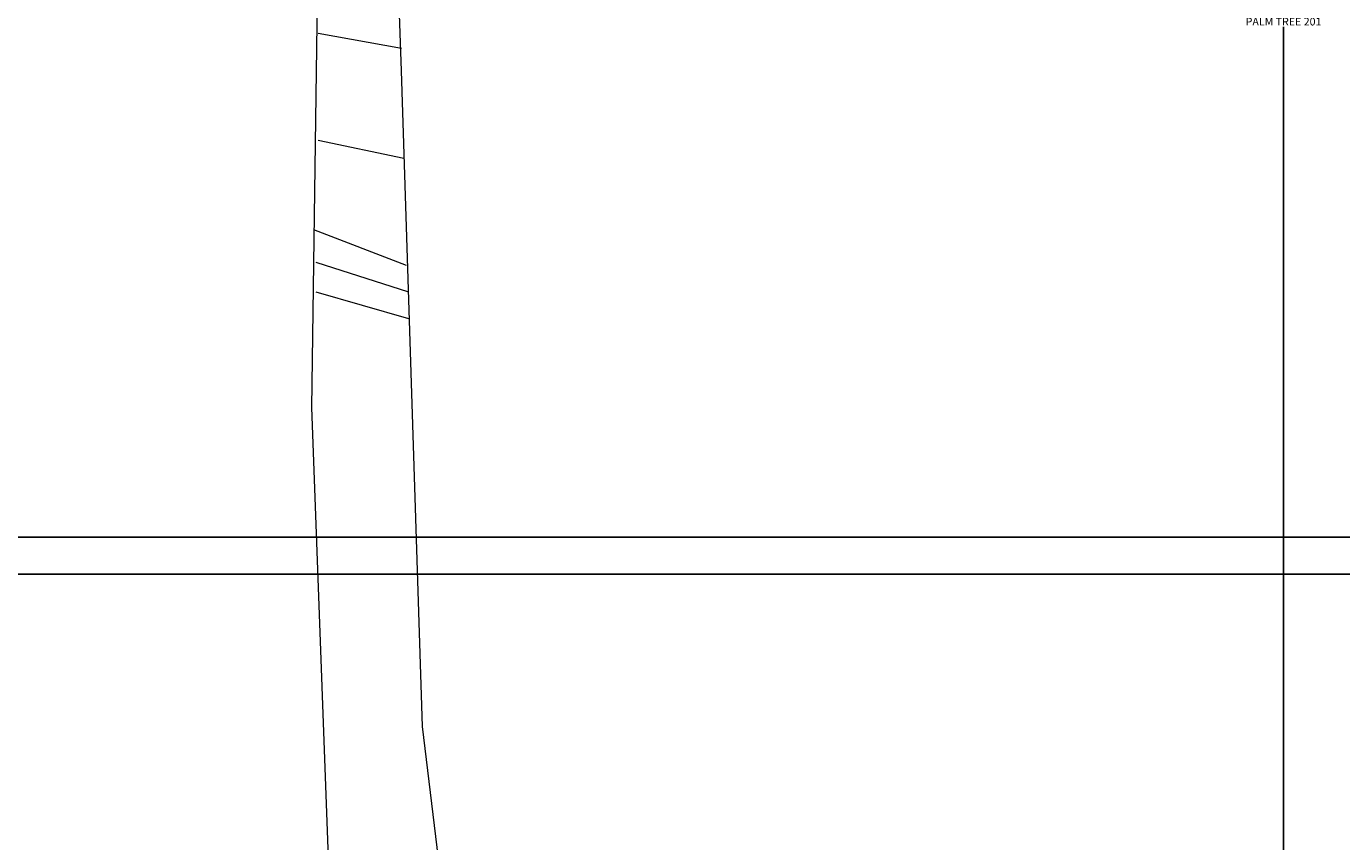
# Model space of a CAD drawing. Units: inches. Extents: x -13 to 809, y 112 to 656.
# Tile 44 of 55: x 641 to 747, y 185 to 251. Entities that reach past the tile are written whole.
import ezdxf

# ---------------------------------------------------------------- set-up
doc = ezdxf.new("R2010")
doc.units = ezdxf.units.IN
doc.header["$MEASUREMENT"] = 0
doc.layers.add('A-ANNO-DIMS', color=2, linetype='Continuous', lineweight=18)
doc.layers.add('L-PLNT', color=3, linetype='Continuous', lineweight=18)
doc.styles.get("Standard").update_dxf_attribs({"font": 'arial.ttf'})
doc.dimstyles.get("Standard").update_dxf_attribs({"dimtxt": 0.625, "dimasz": 0.18, "dimexe": 0.18, "dimexo": 0.0625, "dimgap": 0.09, "dimtad": 0, "dimtih": 1, "dimtoh": 1, "dimdec": 4, "dimzin": 0, "dimdsep": 46, "dimlunit": 4, "dimtxsty": 'Standard', "dimcen": 0.09, "dimadec": 0, "dimazin": 0, "dimtfac": 1, "dimtdec": 4, "dimtofl": 0, "dimtmove": 0, "dimatfit": 3, "dimfxl": 1, "dimtolj": 1, "dimtzin": 0, "dimarcsym": 0})

# ---------------------------------------------------------------- blocks, each defined once
blk = doc.blocks.new('Tree - palm elevation')
for p, q in [((-4.453, 99.651), (2.24, 98.459)), ((-4.453, 91.071), (2.426, 89.641)), ((-4.825, 83.921), (2.612, 81.061)), ((-4.639, 81.299), (2.797, 78.916)), ((-4.639, 78.916), (2.797, 76.771))]:
    blk.add_line(p, q)
for points in [[(-2.363, 170.553), (-3.88, 148.505), (-4.988, 69.634), (-3.325, 24.869), (0, 0)], [(-0.116, 162.848), (0.554, 143.532), (2.217, 96.635), (3.88, 44.054), (7.76, 12.079), (11.64, 0)]]:
    blk.add_lwpolyline(points)
blk = doc.blocks.new('*D9')
at = {"layer": 'A-ANNO-DIMS', "color": 0, "lineweight": -2, "transparency": 16777216}
for p, q in [((711.81, 351.8), (742.1, 351.8)), ((741.92, 351.62), (741.92, 251.63)), ((741.92, 150.81), (741.92, 250.81)), ((711.81, 150.63), (742.1, 150.63))]:
    blk.add_line(p, q, dxfattribs=at)
at = {"layer": 'A-ANNO-DIMS', "color": 0, "transparency": 16777216}
for points in [[(741.89, 351.62), (741.95, 351.62), (741.92, 351.8)], [(741.89, 150.81), (741.95, 150.81), (741.92, 150.63)]]:
    blk.add_solid(points, dxfattribs=at)
at = {"layer": 'Defpoints', "color": 0, "transparency": 16777216}
for p in [(711.75, 351.8), (741.92, 351.8), (711.75, 150.63)]:
    blk.add_point(p, dxfattribs=at)
at = {"layer": 'A-ANNO-DIMS', "color": 0, "transparency": 16777216, "insert": (741.92, 251.22), "char_height": 0.625, "attachment_point": 5}
blk.add_mtext('\\A1;PALM TREE 201', dxfattribs=at)
blk = doc.blocks.new('*D31')
at = {"layer": 'A-ANNO-DIMS', "color": 0, "lineweight": -2, "transparency": 16777216}
for p, q in [((621.07, 617.78), (807.77, 617.78)), ((807.59, 617.6), (807.59, 384.56)), ((807.59, 150.7), (807.59, 383.74)), ((621.07, 150.52), (807.77, 150.52))]:
    blk.add_line(p, q, dxfattribs=at)
at = {"layer": 'A-ANNO-DIMS', "color": 0, "transparency": 16777216}
for points in [[(807.56, 617.6), (807.62, 617.6), (807.59, 617.78)], [(807.56, 150.7), (807.62, 150.7), (807.59, 150.52)]]:
    blk.add_solid(points, dxfattribs=at)
at = {"layer": 'Defpoints', "color": 0, "transparency": 16777216}
for p in [(621.01, 617.78), (807.59, 617.78), (621.01, 150.52)]:
    blk.add_point(p, dxfattribs=at)
at = {"layer": 'A-ANNO-DIMS', "color": 0, "transparency": 16777216, "insert": (807.59, 384.15), "char_height": 0.625, "attachment_point": 5}
blk.add_mtext('\\A1;467.3', dxfattribs=at)
blk = doc.blocks.new('*D129')
at = {"layer": 'A-ANNO-DIMS', "color": 0, "lineweight": -2, "transparency": 16777216}
for p, q in [((607.64, 209.88), (807.77, 209.88)), ((807.59, 209.7), (807.59, 180.61)), ((807.59, 150.7), (807.59, 179.79)), ((608.76, 150.52), (807.77, 150.52))]:
    blk.add_line(p, q, dxfattribs=at)
at = {"layer": 'A-ANNO-DIMS', "color": 0, "transparency": 16777216}
for points in [[(807.56, 209.7), (807.62, 209.7), (807.59, 209.88)], [(807.56, 150.7), (807.62, 150.7), (807.59, 150.52)]]:
    blk.add_solid(points, dxfattribs=at)
at = {"layer": 'Defpoints', "color": 0, "transparency": 16777216}
for p in [(607.57, 209.88), (807.59, 209.88), (608.69, 150.52)]:
    blk.add_point(p, dxfattribs=at)
at = {"layer": 'A-ANNO-DIMS', "color": 0, "transparency": 16777216, "insert": (807.59, 180.2), "char_height": 0.625, "attachment_point": 5}
blk.add_mtext('\\A1;59.36', dxfattribs=at)
blk = doc.blocks.new('*D132')
at = {"layer": 'A-ANNO-DIMS', "color": 0, "lineweight": -2, "transparency": 16777216}
for p, q in [((607.64, 209.88), (807.77, 209.88)), ((807.59, 209.7), (807.59, 208.79)), ((807.59, 207.07), (807.59, 207.97)), ((604.64, 206.89), (807.77, 206.89))]:
    blk.add_line(p, q, dxfattribs=at)
at = {"layer": 'A-ANNO-DIMS', "color": 0, "transparency": 16777216}
for points in [[(807.56, 209.7), (807.62, 209.7), (807.59, 209.88)], [(807.56, 207.07), (807.62, 207.07), (807.59, 206.89)]]:
    blk.add_solid(points, dxfattribs=at)
at = {"layer": 'Defpoints', "color": 0, "transparency": 16777216}
for p in [(607.57, 209.88), (807.59, 209.88), (604.57, 206.89)]:
    blk.add_point(p, dxfattribs=at)
at = {"layer": 'A-ANNO-DIMS', "color": 0, "transparency": 16777216, "insert": (807.59, 208.38), "char_height": 0.625, "attachment_point": 5}
blk.add_mtext('\\A1;2.989', dxfattribs=at)

msp = doc.modelspace()

# ---------------------------------------------------------------- block references
at = {"layer": 'L-PLNT'}
msp.add_blockref('Tree - palm elevation', (668.9925, 150.6343), dxfattribs=at)

# ---------------------------------------------------------------- dimensions: what is measured, and where the dimension line sits
at = {"layer": 'A-ANNO-DIMS'}
for base, p1, p2, override, picture, middle in [((807.5888, 617.7828), (621.008, 150.5199), (621.008, 617.7828), {"dimdec": 1, "dimlfac": 1, "dimrnd": 0, "dimzin": 0, "dimdsep": 46, "dimlunit": 2}, '*D31', (807.5888, 384.1514)), ((807.5888, 209.8753), (604.5741, 206.8866), (607.5741, 209.8753), {"dimdec": 3, "dimlfac": 1, "dimrnd": 0, "dimzin": 0, "dimdsep": 46, "dimlunit": 2}, '*D132', (807.5888, 208.381)), ((807.5888, 209.8753), (608.694, 150.5199), (607.5741, 209.8753), {"dimdec": 2, "dimlfac": 1, "dimrnd": 0, "dimzin": 0, "dimdsep": 46, "dimlunit": 2}, '*D129', (807.5888, 180.1976))]:
    dim = msp.add_linear_dim(base=base, p1=p1, p2=p2, angle=90, dimstyle='Standard', override=override, dxfattribs=at)
    dim.commit()
    dim.dimension.update_dxf_attribs({"geometry": picture, "text_midpoint": middle})
dim = msp.add_linear_dim(base=(741.9246, 351.8013), p1=(711.7495, 150.6343), p2=(711.7495, 351.8013), angle=90, text='PALM TREE <>', dimstyle='Standard', override={"dimdec": 0, "dimlfac": 1, "dimrnd": 0, "dimzin": 0, "dimdsep": 46, "dimlunit": 2}, dxfattribs=at)
dim.commit()
dim.dimension.update_dxf_attribs({"geometry": '*D9', "text_midpoint": (741.9246, 251.2178)})

doc.saveas('drawing.dxf')
